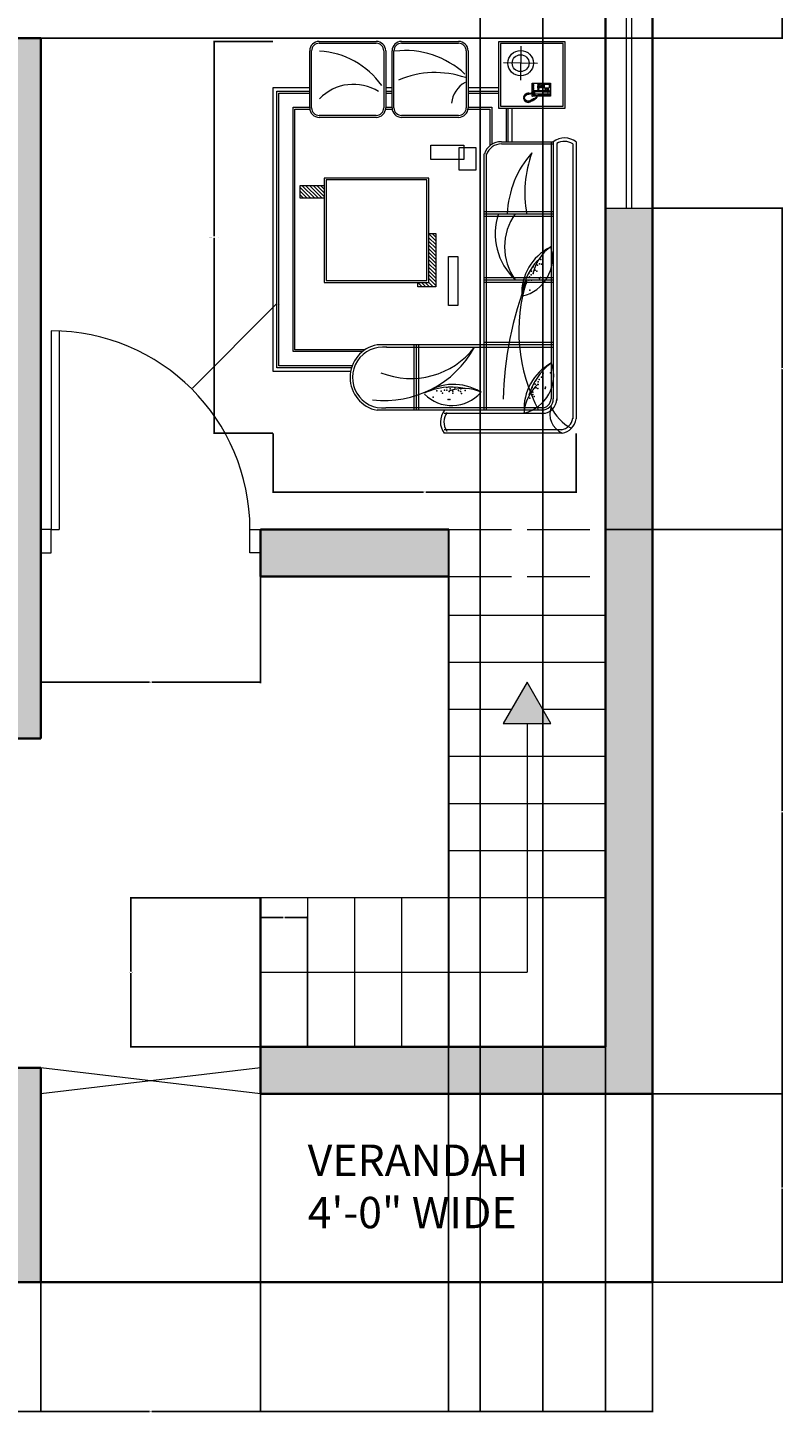
# Model space of a CAD drawing. Units: inches. Extents: x 126 to 477, y -70 to 465.
# Tile 2 of 5: x 332 to 477, y -70 to 195. Entities that reach past the tile are written whole.
import ezdxf

# ---------------------------------------------------------------- set-up
doc = ezdxf.new("R2010")
doc.units = ezdxf.units.IN
doc.linetypes.add('ACAD_ISO02W100', pattern=[15, 12, -3])
for name, color, linetype, lineweight in [('A-ANNO-DIMS', 2, 'Continuous', 18), ('A-ANNO-SYMB', 7, 'Continuous', 18), ('A-AREA-IDEN', 7, 'Continuous', 20), ('A-DOOR', 4, 'Continuous', 20), ('A-DOOR-GATE', 4, 'Continuous', 20), ('A-FLOR-STRS', 7, 'Continuous', 18), ('A-FLOR-STRS-OVHD', 7, 'ACAD_ISO02W100', 18), ('A-FURN', 8, 'Continuous', 18), ('A-GLAZ', 4, 'Continuous', 18), ('A-WALL', 7, 'Continuous', 35), ('A-WALL-PATT', 252, 'Continuous', 13)]:
    doc.layers.add(name, color=color, linetype=linetype, lineweight=lineweight)
doc.styles.get("Standard").update_dxf_attribs({"font": 'arial.ttf'})
doc.dimstyles.get("Standard").update_dxf_attribs({"dimtxt": 0.18, "dimasz": 0.18, "dimexe": 0.18, "dimexo": 0.0625, "dimgap": 0.09, "dimtad": 0, "dimtih": 1, "dimtoh": 1, "dimdec": 4, "dimzin": 0, "dimdsep": 46, "dimtxsty": 'Standard', "dimcen": 0.09, "dimadec": 0, "dimazin": 0, "dimtfac": 1, "dimtdec": 4, "dimtofl": 0, "dimtmove": 0, "dimatfit": 3, "dimfxl": 1, "dimtolj": 1, "dimtzin": 0, "dimarcsym": 0})

# ---------------------------------------------------------------- blocks, each defined once
blk = doc.blocks.new('A$C327A19D4')
for p, q in [((703, 3073), (3, 3073)), ((3, 3073), (3, 2373)), ((703, 2373), (703, 3073)), ((1059, 3191), (3976, 3191)), ((1078, 3155), (3976, 3155)), ((683, 3053), (23, 3053)), ((23, 3053), (23, 2393)), ((683, 2393), (683, 3053)), ((1056, 2949), (3763, 2949)), ((1056, 2403), (1056, 2949)), ((1056, 2925), (3763, 2925)), ((1076, 2985), (3780, 2985)), ((1080, 2403), (1080, 2949)), ((1791, 2223), (1791, 2949)), ((1815, 2465), (1815, 2949)), ((1839, 2223), (1839, 2949)), ((2487, 2223), (2487, 2949)), ((2511, 2223), (2511, 2949)), ((2535, 2223), (2535, 2949)), ((3169, 2223), (3169, 2949)), ((3193, 2465), (3193, 2949)), ((3221, 1195), (3221, 2949)), ((4090, 3043), (4090, 1800)), ((4126, 3043), (4126, 1800)), ((231, 2784), (227, 2425)), ((1815, 2223), (1815, 2872)), ((1815, 2223), (1815, 2872)), ((1815, 2465), (1815, 2872)), ((1815, 2465), (1815, 2872)), ((3193, 2223), (3193, 2872)), ((3193, 2223), (3193, 2872)), ((3193, 2465), (3193, 2872)), ((3193, 2465), (3193, 2872)), ((3860, 2828), (3860, 1185)), ((3884, 2828), (3884, 1095)), ((3920, 2867), (3920, 1802)), ((49, 2607), (409, 2603)), ((703, 2512), (1056, 2512)), ((3, 2373), (703, 2373)), ((23, 2393), (683, 2393)), ((484, 2052), (484, 2373)), ((524, 2052), (524, 2373)), ((544, 2052), (544, 2373)), ((703, 2472), (1056, 2472)), ((703, 2452), (1056, 2452)), ((694, 2052), (694, 2302)), ((694, 2302), (1084, 2302)), ((714, 2051), (714, 2282)), ((714, 2282), (1098, 2282)), ((3884, 2247), (1184, 2247)), ((3884, 2223), (1184, 2223)), ((3195, 2235), (3195, 1095)), ((1119, 2135), (1357, 2135)), ((1119, 1958), (1119, 2135)), ((1357, 2135), (1357, 1958)), ((1092, 2007), (1244, 2007)), ((1092, 1659), (1092, 2007)), ((1357, 1958), (1119, 1958)), ((1244, 2007), (1244, 1659)), ((2265, 1945), (2780, 1945)), ((2265, 1845), (2265, 1945)), ((2780, 1945), (2780, 1845)), ((2780, 1845), (2265, 1845)), ((1244, 1659), (1092, 1659)), ((2539, 1638), (1439, 1638)), ((1439, 1638), (1439, 538)), ((2519, 1618), (1459, 1618)), ((1459, 1618), (1459, 558)), ((2023, 1638), (2023, 1711)), ((2023, 1711), (2585, 1711)), ((2519, 558), (2519, 1618)), ((2539, 538), (2539, 1638)), ((2585, 1711), (2585, 1522)), ((2585, 1522), (2539, 1522)), ((3884, 1532), (3195, 1532)), ((3884, 1508), (3195, 1508)), ((3884, 1484), (3195, 1484)), ((484, 1185), (484, 1252)), ((524, 1185), (524, 1252)), ((544, 1185), (544, 1252)), ((694, 1185), (694, 1252)), ((714, 1184), (714, 1253)), ((3247, 967), (3247, 230)), ((3267, 940), (3267, 210)), ((3417, 832), (3417, 60)), ((3437, 825), (3437, 40)), ((3477, 816), (3477, 0)), ((1439, 538), (2539, 538)), ((1459, 558), (2519, 558)), ((1516, 538), (1651, 538)), ((1516, 285), (1516, 538)), ((1651, 538), (1651, 285)), ((484, 0), (484, 385)), ((524, 40), (524, 385)), ((544, 60), (544, 385)), ((694, 210), (694, 385)), ((714, 230), (714, 386)), ((3267, 210), (694, 210)), ((3247, 230), (714, 230)), ((1651, 285), (1516, 285)), ((3437, 40), (524, 40)), ((3417, 60), (544, 60)), ((3477, 0), (484, 0))]:
    blk.add_line(p, q)
at = {"linetype": 'ByBlock'}
for p, q in [((438, 2915), (440, 2918)), ((440, 2918), (576, 2919)), ((576, 2919), (578, 2916)), ((439, 2728), (438, 2915)), ((451, 2906), (490, 2906)), ((451, 2856), (451, 2906)), ((491, 2856), (451, 2856)), ((453, 2831), (453, 2839)), ((453, 2839), (461, 2839)), ((461, 2831), (453, 2831)), ((453, 2824), (461, 2825)), ((453, 2816), (453, 2824)), ((461, 2816), (453, 2816)), ((453, 2801), (453, 2810)), ((453, 2810), (461, 2810)), ((461, 2802), (453, 2801)), ((453, 2787), (453, 2795)), ((453, 2795), (461, 2795)), ((461, 2787), (453, 2787)), ((461, 2839), (461, 2831)), ((461, 2825), (461, 2816)), ((461, 2810), (461, 2802)), ((461, 2795), (461, 2787)), ((466, 2839), (475, 2840)), ((467, 2831), (466, 2839)), ((475, 2831), (467, 2831)), ((467, 2816), (467, 2825)), ((467, 2825), (475, 2825)), ((475, 2817), (467, 2816)), ((467, 2802), (467, 2810)), ((467, 2810), (475, 2810)), ((475, 2802), (467, 2802)), ((467, 2787), (467, 2795)), ((467, 2795), (475, 2795)), ((475, 2787), (467, 2787)), ((475, 2840), (475, 2831)), ((475, 2825), (475, 2817)), ((475, 2810), (475, 2802)), ((475, 2795), (475, 2787)), ((480, 2840), (488, 2840)), ((480, 2831), (480, 2840)), ((488, 2832), (480, 2831)), ((480, 2817), (480, 2825)), ((480, 2825), (488, 2825)), ((488, 2817), (480, 2817)), ((480, 2810), (488, 2810)), ((480, 2802), (480, 2810)), ((488, 2802), (480, 2802)), ((480, 2787), (480, 2795)), ((480, 2795), (488, 2795)), ((488, 2787), (480, 2787)), ((488, 2840), (488, 2832)), ((488, 2825), (488, 2817)), ((488, 2810), (488, 2802)), ((488, 2795), (488, 2787)), ((490, 2906), (491, 2856)), ((505, 2903), (494, 2903)), ((494, 2903), (494, 2899)), ((494, 2899), (505, 2899)), ((495, 2895), (495, 2891)), ((505, 2895), (495, 2895)), ((495, 2891), (505, 2891)), ((495, 2887), (495, 2883)), ((505, 2887), (495, 2887)), ((495, 2883), (505, 2883)), ((495, 2879), (495, 2875)), ((505, 2879), (495, 2879)), ((495, 2875), (505, 2875)), ((495, 2871), (495, 2867)), ((506, 2871), (495, 2871)), ((495, 2867), (506, 2867)), ((495, 2863), (495, 2859)), ((506, 2863), (495, 2863)), ((495, 2859), (506, 2859)), ((497, 2795), (507, 2795)), ((497, 2787), (497, 2795)), ((507, 2787), (497, 2787)), ((505, 2899), (505, 2903)), ((505, 2891), (505, 2895)), ((505, 2883), (505, 2887)), ((505, 2875), (505, 2879)), ((506, 2867), (506, 2871)), ((506, 2859), (506, 2863)), ((507, 2795), (507, 2787)), ((515, 2908), (520, 2914)), ((516, 2744), (515, 2908)), ((520, 2910), (519, 2905)), ((519, 2905), (531, 2893)), ((519, 2905), (519, 2868)), ((519, 2868), (522, 2862)), ((520, 2914), (561, 2915)), ((526, 2913), (520, 2910)), ((520, 2783), (522, 2790)), ((520, 2746), (520, 2783)), ((522, 2862), (526, 2855)), ((522, 2790), (526, 2797)), ((532, 2895), (526, 2913)), ((526, 2913), (558, 2913)), ((526, 2855), (527, 2845)), ((526, 2797), (528, 2806)), ((527, 2845), (527, 2832)), ((528, 2806), (527, 2832)), ((531, 2893), (532, 2895)), ((532, 2832), (531, 2893)), ((551, 2896), (532, 2895)), ((532, 2832), (532, 2759)), ((551, 2896), (558, 2913)), ((553, 2893), (551, 2896)), ((565, 2905), (553, 2893)), ((553, 2832), (553, 2893)), ((553, 2832), (554, 2759)), ((558, 2855), (557, 2846)), ((557, 2846), (557, 2832)), ((557, 2806), (557, 2832)), ((559, 2797), (557, 2806)), ((558, 2913), (563, 2911)), ((562, 2862), (558, 2855)), ((563, 2790), (559, 2797)), ((561, 2915), (568, 2908)), ((565, 2869), (562, 2862)), ((563, 2911), (565, 2905)), ((566, 2783), (563, 2790)), ((565, 2905), (565, 2869)), ((566, 2747), (566, 2783)), ((568, 2908), (569, 2745)), ((578, 2916), (580, 2729)), ((587, 2779), (579, 2779)), ((579, 2775), (584, 2774)), ((584, 2774), (587, 2772)), ((590, 2777), (587, 2779)), ((587, 2772), (591, 2770)), ((594, 2771), (590, 2777)), ((599, 2771), (594, 2771)), ((602, 2770), (599, 2771)), ((442, 2726), (439, 2728)), ((543, 2726), (442, 2726)), ((468, 2743), (455, 2743)), ((455, 2743), (455, 2735)), ((455, 2735), (469, 2735)), ((469, 2735), (468, 2743)), ((487, 2743), (474, 2743)), ((474, 2743), (474, 2735)), ((474, 2735), (487, 2735)), ((487, 2735), (487, 2743)), ((493, 2744), (493, 2735)), ((506, 2744), (493, 2744)), ((493, 2735), (506, 2735)), ((506, 2735), (506, 2744)), ((523, 2737), (516, 2744)), ((520, 2746), (532, 2759)), ((521, 2741), (520, 2746)), ((527, 2738), (521, 2741)), ((542, 2737), (523, 2737)), ((533, 2756), (527, 2738)), ((527, 2738), (542, 2738)), ((532, 2759), (533, 2756)), ((552, 2756), (533, 2756)), ((546, 2743), (542, 2743)), ((542, 2743), (542, 2731)), ((542, 2731), (545, 2717)), ((545, 2717), (549, 2704)), ((547, 2732), (546, 2743)), ((546, 2738), (559, 2739)), ((562, 2737), (546, 2737)), ((549, 2696), (546, 2692)), ((546, 2692), (546, 2686)), ((546, 2686), (554, 2685)), ((554, 2685), (546, 2680)), ((546, 2680), (547, 2672)), ((548, 2723), (547, 2732)), ((547, 2672), (555, 2672)), ((577, 2726), (548, 2726)), ((552, 2710), (548, 2723)), ((549, 2704), (548, 2697)), ((548, 2697), (549, 2696)), ((555, 2672), (548, 2666)), ((548, 2666), (551, 2659)), ((551, 2659), (560, 2661)), ((554, 2759), (552, 2756)), ((552, 2756), (559, 2739)), ((553, 2703), (552, 2710)), ((552, 2696), (553, 2703)), ((557, 2693), (552, 2696)), ((566, 2747), (554, 2759)), ((556, 2687), (557, 2693)), ((558, 2669), (556, 2687)), ((560, 2661), (556, 2653)), ((556, 2653), (560, 2648)), ((568, 2656), (558, 2669)), ((559, 2739), (565, 2741)), ((560, 2648), (566, 2653)), ((569, 2745), (562, 2737)), ((565, 2741), (566, 2747)), ((566, 2653), (565, 2646)), ((565, 2646), (570, 2642)), ((583, 2649), (568, 2656)), ((570, 2642), (577, 2648)), ((577, 2648), (576, 2639)), ((576, 2639), (582, 2637)), ((580, 2729), (577, 2726)), ((582, 2637), (585, 2645)), ((599, 2647), (583, 2649)), ((585, 2645), (589, 2637)), ((589, 2637), (593, 2637)), ((591, 2770), (593, 2768)), ((595, 2768), (592, 2765)), ((592, 2765), (597, 2757)), ((593, 2768), (595, 2768)), ((593, 2637), (595, 2645)), ((595, 2645), (598, 2636)), ((597, 2757), (606, 2742)), ((598, 2636), (604, 2637)), ((599, 2760), (603, 2767)), ((606, 2763), (599, 2760)), ((615, 2654), (599, 2647)), ((603, 2767), (602, 2770)), ((604, 2750), (608, 2758)), ((612, 2753), (604, 2750)), ((604, 2645), (610, 2639)), ((604, 2637), (604, 2645)), ((608, 2758), (606, 2763)), ((606, 2742), (612, 2731)), ((608, 2742), (614, 2749)), ((615, 2746), (608, 2742)), ((610, 2639), (615, 2642)), ((614, 2749), (612, 2753)), ((612, 2731), (614, 2730)), ((613, 2733), (618, 2740)), ((621, 2736), (613, 2733)), ((614, 2730), (613, 2728)), ((613, 2728), (622, 2712)), ((614, 2650), (619, 2643)), ((615, 2642), (614, 2650)), ((618, 2740), (615, 2746)), ((627, 2666), (615, 2654)), ((619, 2643), (624, 2647)), ((620, 2723), (624, 2730)), ((627, 2725), (620, 2723)), ((620, 2654), (628, 2651)), ((624, 2647), (620, 2654)), ((624, 2730), (621, 2736)), ((622, 2712), (631, 2687)), ((626, 2712), (630, 2720)), ((634, 2713), (626, 2712)), ((630, 2720), (627, 2725)), ((631, 2687), (627, 2666)), ((628, 2702), (636, 2705)), ((637, 2702), (628, 2702)), ((628, 2661), (636, 2659)), ((632, 2654), (628, 2661)), ((628, 2651), (632, 2654)), ((631, 2672), (640, 2672)), ((638, 2665), (631, 2672)), ((633, 2691), (639, 2696)), ((641, 2691), (633, 2691)), ((636, 2705), (634, 2713)), ((634, 2681), (642, 2684)), ((641, 2677), (634, 2681)), ((636, 2659), (638, 2665)), ((639, 2696), (637, 2702)), ((640, 2672), (641, 2677)), ((642, 2684), (641, 2691))]:
    blk.add_line(p, q, dxfattribs=at)
at = {"ltscale": 5}
for p, q in [((100, 2052), (700, 2052)), ((0, 1352), (0, 1952)), ((20, 1352), (20, 1952)), ((100, 2032), (700, 2032)), ((780, 1952), (780, 1352)), ((800, 1952), (800, 1352)), ((2023, 1673), (2061, 1711)), ((2027, 1638), (2100, 1711)), ((2067, 1638), (2139, 1711)), ((2106, 1638), (2179, 1711)), ((2145, 1638), (2218, 1711)), ((2184, 1638), (2257, 1711)), ((2224, 1638), (2296, 1711)), ((2263, 1638), (2336, 1711)), ((2302, 1638), (2375, 1711)), ((2341, 1638), (2414, 1711)), ((2381, 1638), (2453, 1711)), ((2420, 1638), (2493, 1711)), ((2459, 1638), (2532, 1711)), ((2498, 1638), (2571, 1711)), ((2538, 1638), (2585, 1685)), ((2539, 1601), (2585, 1646)), ((2539, 1561), (2585, 1607)), ((2539, 1522), (2585, 1568)), ((2578, 1522), (2585, 1528)), ((700, 1272), (100, 1272)), ((700, 1252), (100, 1252)), ((100, 1185), (700, 1185)), ((0, 485), (0, 1085)), ((20, 485), (20, 1085)), ((100, 1165), (700, 1165)), ((780, 1085), (780, 485)), ((800, 1085), (800, 485)), ((1516, 499), (1555, 538)), ((1516, 460), (1594, 538)), ((1516, 421), (1634, 538)), ((1516, 382), (1651, 516)), ((1516, 342), (1651, 477)), ((1516, 303), (1651, 438)), ((700, 405), (100, 405)), ((700, 385), (100, 385)), ((1537, 285), (1651, 398)), ((1576, 285), (1651, 359)), ((1616, 285), (1651, 320))]:
    blk.add_line(p, q, dxfattribs=at)
for radius in [134, 88.7]:
    blk.add_circle((229, 2605), radius)
for centre, radius, start, end in [((1218, 3068), 201, 142.4201, 216.3682), ((1218, 3068), 165, 148.4003, 210.2229), ((3657, 3353), 468, 293.6733, 332.9672), ((3943, 3007), 150, 10.9855, 79.893), ((3943, 3007), 187, 10.9855, 79.893), ((2545, 3192), 468, 214.7097, 257.8799), ((2283, 2531), 409, 13.4523, 105.9639), ((3869, 3188), 547, 208.8478, 273.48), ((3911, 3323), 657, 217.6007, 253.5739), ((3517, 2544), 409, 14.6876, 107.1992), ((3763, 2828), 157, 0, 90), ((3763, 2828), 121, 0, 90), ((3763, 2828), 96.8, 0, 90), ((3921, 3138), 226, 250.4844, 335.1673), ((2657, 3163), 547, 207.1715, 271.8037), ((2752, 3267), 657, 227.0776, 263.0508), ((3052, 4350), 1764, 252.1519, 298.1592), ((3951, 3106), 468, 222.7716, 265.9418), ((1594, 3859), 1211, 249.7283, 280.5443), ((1853, 3485), 1021, 228.2765, 267.8541), ((3865, 6197), 3777, 248.9971, 268.5461), ((2024, 3008), 670, 251.8392, 316.629), ((2163, 3036), 599, 234.5154, 305.4846), ((1243, 2401), 187, 179.2584, 251.6848), ((1243, 2401), 163, 179.2584, 251.6848), ((4124, 2008), 468, 156.691, 199.8613), ((4159, 1898), 547, 149.1529, 213.7851), ((3425, 1881), 409, 315.4337, 47.9453), ((4298, 1873), 657, 169.059, 205.0321), ((4007, 1962), 201, 232.4201, 306.3682), ((4007, 1962), 165, 232.4201, 306.3682)]:
    blk.add_arc(centre, radius, start, end)
for centre, radius, start, end in [((100, 1952), 100, 90, 180), ((700, 1952), 100, 0, 90), ((100, 1952), 80, 90, 180), ((1024, 1388), 928, 137.1341, 186.5635), ((1307, 1706), 979, 160.9364, 203.1944), ((676, 2156), 279, 209.1633, 264.4137), ((700, 1952), 80, 0, 90), ((100, 1352), 100, 180, 270), ((100, 1352), 80, 180, 270), ((700, 1352), 80, 270, 0), ((700, 1352), 100, 270, 0), ((100, 1085), 100, 90, 180), ((700, 1085), 100, 0, 90), ((100, 1085), 80, 90, 180), ((968, 436), 868, 125.4807, 176.5616), ((949, 846), 497, 147.8484, 226.1244), ((700, 1085), 80, 0, 90), ((100, 485), 100, 180, 270), ((100, 485), 80, 180, 270), ((700, 485), 100, 270, 0), ((700, 485), 80, 270, 0)]:
    blk.add_arc(centre, radius, start, end, dxfattribs=at)
at = {"ltscale": 20}
for centre, radius, start, end in [((2701, 1449), 849, 338.2682, 52.2695), ((2703, 1175), 1078, 353.1988, 61.2564), ((3540, 1156), 321, 172.9078, 5.2194), ((3540, 1161), 351, 190.8398, 349.1602)]:
    blk.add_arc(centre, radius, start, end, dxfattribs=at)
for p in [(3492, 2920), (2298, 2818), (2329, 2780), (2344, 2802), (2345, 2825), (2356, 2781), (2421, 2774), (2485, 2814), (2498, 2803), (3495, 2842), (3535, 2825), (3560, 2838), (3561, 2800), (3585, 2789), (3612, 2788), (3641, 2868), (3655, 2787), (3657, 2862), (2375, 2736), (2410, 2757), (2421, 2720), (2444, 2738), (2445, 2691), (2459, 2715), (2481, 2700), (2514, 2718), (2515, 2690), (2551, 2664), (2620, 2701), (3571, 2765), (3609, 2758), (3646, 2728), (3647, 2768), (3694, 2735), (3707, 2710), (3719, 2734), (3738, 2747), (3756, 2703), (3648, 1911), (3660, 1974), (3676, 1951), (3677, 2020), (3687, 1973), (3707, 1984), (3646, 1828), (3658, 1864), (3673, 1803), (3674, 1829), (3683, 1768), (3684, 1893), (3686, 1853), (3705, 1892), (3706, 1784), (3770, 1842), (3772, 1859), (3680, 1724), (3748, 1685)]:
    blk.add_point(p)
blk = doc.blocks.new('WIN-72IN')
for p, q in [((0, 0), (0, 9)), ((72, 0), (72, 9)), ((72, 5), (0, 5)), ((72, 4), (0, 4))]:
    blk.add_line(p, q)
blk = doc.blocks.new('*D25')
at = {"layer": 'A-ANNO-DIMS', "color": 0, "lineweight": -2, "transparency": 16777216}
for p, q in [((378.9, 192.26), (367.54, 192.26)), ((367.72, 192.08), (367.72, 154.96)), ((367.72, 117.47), (367.72, 154.59)), ((378.9, 117.29), (367.54, 117.29))]:
    blk.add_line(p, q, dxfattribs=at)
at = {"layer": 'A-ANNO-DIMS', "color": 0, "transparency": 16777216}
for points in [[(367.69, 192.08), (367.75, 192.08), (367.72, 192.26)], [(367.69, 117.47), (367.75, 117.47), (367.72, 117.29)]]:
    blk.add_solid(points, dxfattribs=at)
at = {"layer": 'Defpoints', "color": 0, "transparency": 16777216}
for p in [(378.96, 192.26), (367.72, 117.29), (378.96, 117.29)]:
    blk.add_point(p, dxfattribs=at)
at = {"layer": 'A-ANNO-DIMS', "color": 0, "transparency": 16777216, "insert": (367.72, 154.77), "char_height": 0.18, "attachment_point": 5}
blk.add_mtext('\\A1;LOUNGE SET 75', dxfattribs=at)
blk = doc.blocks.new('*D26')
at = {"layer": 'A-ANNO-DIMS', "color": 0, "lineweight": -2, "transparency": 16777216}
for p, q in [((378.96, 117.23), (378.96, 105.86)), ((436.94, 117.23), (436.94, 105.86)), ((379.14, 106.04), (407.73, 106.04)), ((436.76, 106.04), (408.17, 106.04))]:
    blk.add_line(p, q, dxfattribs=at)
at = {"layer": 'A-ANNO-DIMS', "color": 0, "transparency": 16777216}
for points in [[(379.14, 106.07), (379.14, 106.01), (378.96, 106.04)], [(436.76, 106.07), (436.76, 106.01), (436.94, 106.04)]]:
    blk.add_solid(points, dxfattribs=at)
at = {"layer": 'Defpoints', "color": 0, "transparency": 16777216}
for p in [(378.96, 117.29), (436.94, 117.29), (436.94, 106.04)]:
    blk.add_point(p, dxfattribs=at)
at = {"layer": 'A-ANNO-DIMS', "color": 0, "transparency": 16777216, "insert": (407.95, 106.04), "char_height": 0.18, "attachment_point": 5}
blk.add_mtext('\\A1;58', dxfattribs=at)
blk = doc.blocks.new('*D32')
at = {"layer": 'A-ANNO-DIMS', "color": 0, "lineweight": -2, "transparency": 16777216}
for p, q in [((430.53, 430.82), (430.53, -70.05)), ((442.53, 430.82), (442.53, -70.05)), ((430.71, -69.87), (436.32, -69.87)), ((442.35, -69.87), (436.74, -69.87))]:
    blk.add_line(p, q, dxfattribs=at)
at = {"layer": 'A-ANNO-DIMS', "color": 0, "transparency": 16777216}
for points in [[(430.71, -69.84), (430.71, -69.9), (430.53, -69.87)], [(442.35, -69.84), (442.35, -69.9), (442.53, -69.87)]]:
    blk.add_solid(points, dxfattribs=at)
at = {"layer": 'Defpoints', "color": 0, "transparency": 16777216}
for p in [(430.53, 430.88), (442.53, 430.88), (442.53, -69.87)]:
    blk.add_point(p, dxfattribs=at)
at = {"layer": 'A-ANNO-DIMS', "color": 0, "transparency": 16777216, "insert": (436.53, -69.87), "char_height": 0.18, "attachment_point": 5}
blk.add_mtext('\\A1;12', dxfattribs=at)
blk = doc.blocks.new('*D34')
at = {"layer": 'A-ANNO-DIMS', "color": 0, "lineweight": -2, "transparency": 16777216}
for p, q in [((451.6, -9.12), (476.46, -9.12)), ((476.28, -9.3), (476.28, -26.94)), ((476.28, -44.94), (476.28, -27.3)), ((451.6, -45.12), (476.46, -45.12))]:
    blk.add_line(p, q, dxfattribs=at)
at = {"layer": 'A-ANNO-DIMS', "color": 0, "transparency": 16777216}
for points in [[(476.25, -9.3), (476.31, -9.3), (476.28, -9.12)], [(476.25, -44.94), (476.31, -44.94), (476.28, -45.12)]]:
    blk.add_solid(points, dxfattribs=at)
at = {"layer": 'Defpoints', "color": 0, "transparency": 16777216}
for p in [(451.53, -9.12), (476.28, -9.12), (451.53, -45.12)]:
    blk.add_point(p, dxfattribs=at)
at = {"layer": 'A-ANNO-DIMS', "color": 0, "transparency": 16777216, "insert": (476.28, -27.12), "char_height": 0.18, "attachment_point": 5}
blk.add_mtext('\\A1;36', dxfattribs=at)
blk = doc.blocks.new('*D35')
at = {"layer": 'A-ANNO-DIMS', "color": 0, "lineweight": -2, "transparency": 16777216}
for p, q in [((442.6, 98.88), (476.46, 98.88)), ((476.28, 98.7), (476.28, 45.06)), ((476.28, -8.94), (476.28, 44.7)), ((451.6, -9.12), (476.46, -9.12))]:
    blk.add_line(p, q, dxfattribs=at)
at = {"layer": 'A-ANNO-DIMS', "color": 0, "transparency": 16777216}
for points in [[(476.25, 98.7), (476.31, 98.7), (476.28, 98.88)], [(476.25, -8.94), (476.31, -8.94), (476.28, -9.12)]]:
    blk.add_solid(points, dxfattribs=at)
at = {"layer": 'Defpoints', "color": 0, "transparency": 16777216}
for p in [(442.53, 98.88), (476.28, 98.88), (451.53, -9.12)]:
    blk.add_point(p, dxfattribs=at)
at = {"layer": 'A-ANNO-DIMS', "color": 0, "transparency": 16777216, "insert": (476.28, 44.88), "char_height": 0.18, "attachment_point": 5}
blk.add_mtext('\\A1;108', dxfattribs=at)
blk = doc.blocks.new('*D36')
at = {"layer": 'A-ANNO-DIMS', "color": 0, "lineweight": -2, "transparency": 16777216}
for p, q in [((451.6, 160.38), (476.46, 160.38)), ((476.28, 160.2), (476.28, 129.81)), ((476.28, 99.06), (476.28, 129.45)), ((442.6, 98.88), (476.46, 98.88))]:
    blk.add_line(p, q, dxfattribs=at)
at = {"layer": 'A-ANNO-DIMS', "color": 0, "transparency": 16777216}
for points in [[(476.25, 160.2), (476.31, 160.2), (476.28, 160.38)], [(476.25, 99.06), (476.31, 99.06), (476.28, 98.88)]]:
    blk.add_solid(points, dxfattribs=at)
at = {"layer": 'Defpoints', "color": 0, "transparency": 16777216}
for p in [(451.53, 160.38), (476.28, 160.38), (442.53, 98.88)]:
    blk.add_point(p, dxfattribs=at)
at = {"layer": 'A-ANNO-DIMS', "color": 0, "transparency": 16777216, "insert": (476.28, 129.63), "char_height": 0.18, "attachment_point": 5}
blk.add_mtext('\\A1;61.5', dxfattribs=at)
blk = doc.blocks.new('*D40')
at = {"layer": 'A-ANNO-DIMS', "color": 0, "lineweight": -2, "transparency": 16777216}
for p, q in [((317.53, -45.18), (317.53, -70.05)), ((334.53, -45.18), (334.53, -70.05)), ((317.71, -69.87), (325.82, -69.87)), ((334.35, -69.87), (326.24, -69.87))]:
    blk.add_line(p, q, dxfattribs=at)
at = {"layer": 'A-ANNO-DIMS', "color": 0, "transparency": 16777216}
for points in [[(317.71, -69.84), (317.71, -69.9), (317.53, -69.87)], [(334.35, -69.84), (334.35, -69.9), (334.53, -69.87)]]:
    blk.add_solid(points, dxfattribs=at)
at = {"layer": 'Defpoints', "color": 0, "transparency": 16777216}
for p in [(317.53, -45.12), (334.53, -45.12), (334.53, -69.87)]:
    blk.add_point(p, dxfattribs=at)
at = {"layer": 'A-ANNO-DIMS', "color": 0, "transparency": 16777216, "insert": (326.03, -69.87), "char_height": 0.18, "attachment_point": 5}
blk.add_mtext('\\A1;17', dxfattribs=at)
blk = doc.blocks.new('*D41')
at = {"layer": 'A-ANNO-DIMS', "color": 0, "lineweight": -2, "transparency": 16777216}
for p, q in [((334.53, -4.18), (334.53, -70.05)), ((376.53, -9.18), (376.53, -70.05)), ((334.71, -69.87), (355.31, -69.87)), ((376.35, -69.87), (355.75, -69.87))]:
    blk.add_line(p, q, dxfattribs=at)
at = {"layer": 'A-ANNO-DIMS', "color": 0, "transparency": 16777216}
for points in [[(334.71, -69.84), (334.71, -69.9), (334.53, -69.87)], [(376.35, -69.84), (376.35, -69.9), (376.53, -69.87)]]:
    blk.add_solid(points, dxfattribs=at)
at = {"layer": 'Defpoints', "color": 0, "transparency": 16777216}
for p in [(334.53, -4.12), (376.53, -9.12), (376.53, -69.87)]:
    blk.add_point(p, dxfattribs=at)
at = {"layer": 'A-ANNO-DIMS', "color": 0, "transparency": 16777216, "insert": (355.53, -69.87), "char_height": 0.18, "attachment_point": 5}
blk.add_mtext('\\A1;42', dxfattribs=at)
blk = doc.blocks.new('*D42')
at = {"layer": 'A-ANNO-DIMS', "color": 0, "lineweight": -2, "transparency": 16777216}
for p, q in [((376.53, -9.18), (376.53, -70.05)), ((451.53, -9.18), (451.53, -70.05)), ((376.71, -69.87), (413.81, -69.87)), ((451.35, -69.87), (414.25, -69.87))]:
    blk.add_line(p, q, dxfattribs=at)
at = {"layer": 'A-ANNO-DIMS', "color": 0, "transparency": 16777216}
for points in [[(376.71, -69.84), (376.71, -69.9), (376.53, -69.87)], [(451.35, -69.84), (451.35, -69.9), (451.53, -69.87)]]:
    blk.add_solid(points, dxfattribs=at)
at = {"layer": 'Defpoints', "color": 0, "transparency": 16777216}
for p in [(376.53, -9.12), (451.53, -9.12), (451.53, -69.87)]:
    blk.add_point(p, dxfattribs=at)
at = {"layer": 'A-ANNO-DIMS', "color": 0, "transparency": 16777216, "insert": (414.03, -69.87), "char_height": 0.18, "attachment_point": 5}
blk.add_mtext('\\A1;75', dxfattribs=at)
blk = doc.blocks.new('*D43')
at = {"layer": 'A-ANNO-DIMS', "color": 0, "lineweight": -2, "transparency": 16777216}
for p, q in [((412.53, 98.82), (412.53, -70.05)), ((442.53, 98.82), (442.53, -70.05)), ((412.71, -69.87), (427.31, -69.87)), ((442.35, -69.87), (427.75, -69.87))]:
    blk.add_line(p, q, dxfattribs=at)
at = {"layer": 'A-ANNO-DIMS', "color": 0, "transparency": 16777216}
for points in [[(412.71, -69.84), (412.71, -69.9), (412.53, -69.87)], [(442.35, -69.84), (442.35, -69.9), (442.53, -69.87)]]:
    blk.add_solid(points, dxfattribs=at)
at = {"layer": 'Defpoints', "color": 0, "transparency": 16777216}
for p in [(412.53, 98.88), (442.53, 98.88), (442.53, -69.87)]:
    blk.add_point(p, dxfattribs=at)
at = {"layer": 'A-ANNO-DIMS', "color": 0, "transparency": 16777216, "insert": (427.53, -69.87), "char_height": 0.18, "attachment_point": 5}
blk.add_mtext('\\A1;30', dxfattribs=at)
blk = doc.blocks.new('*D44')
at = {"layer": 'A-ANNO-DIMS', "color": 0, "lineweight": -2, "transparency": 16777216}
for p, q in [((376.47, 28.4), (351.6, 28.4)), ((351.78, 28.22), (351.78, 14.32)), ((351.78, 0.06), (351.78, 13.96)), ((376.47, -0.12), (351.6, -0.12))]:
    blk.add_line(p, q, dxfattribs=at)
at = {"layer": 'A-ANNO-DIMS', "color": 0, "transparency": 16777216}
for points in [[(351.75, 28.22), (351.81, 28.22), (351.78, 28.4)], [(351.75, 0.06), (351.81, 0.06), (351.78, -0.12)]]:
    blk.add_solid(points, dxfattribs=at)
at = {"layer": 'Defpoints', "color": 0, "transparency": 16777216}
for p in [(351.78, 28.4), (376.53, 28.4), (376.53, -0.12)]:
    blk.add_point(p, dxfattribs=at)
at = {"layer": 'A-ANNO-DIMS', "color": 0, "transparency": 16777216, "insert": (351.78, 14.14), "char_height": 0.18, "attachment_point": 5}
blk.add_mtext('\\A1;28.524', dxfattribs=at)
blk = doc.blocks.new('*D45')
at = {"layer": 'A-ANNO-DIMS', "color": 0, "lineweight": -2, "transparency": 16777216}
for p, q in [((376.53, -0.06), (376.53, 24.81)), ((376.71, 24.63), (380.88, 24.63)), ((385.35, 24.63), (381.18, 24.63)), ((385.53, -0.06), (385.53, 24.81))]:
    blk.add_line(p, q, dxfattribs=at)
at = {"layer": 'A-ANNO-DIMS', "color": 0, "transparency": 16777216}
for points in [[(376.71, 24.66), (376.71, 24.6), (376.53, 24.63)], [(385.35, 24.66), (385.35, 24.6), (385.53, 24.63)]]:
    blk.add_solid(points, dxfattribs=at)
at = {"layer": 'Defpoints', "color": 0, "transparency": 16777216}
for p in [(385.53, 24.63), (376.53, -0.12), (385.53, -0.12)]:
    blk.add_point(p, dxfattribs=at)
at = {"layer": 'A-ANNO-DIMS', "color": 0, "transparency": 16777216, "insert": (381.03, 24.63), "char_height": 0.18, "attachment_point": 5}
blk.add_mtext('\\A1;9', dxfattribs=at)
blk = doc.blocks.new('*D47')
at = {"layer": 'A-ANNO-DIMS', "color": 0, "lineweight": -2, "transparency": 16777216}
for p, q in [((334.53, 94.32), (334.53, 69.45)), ((376.53, 94.32), (376.53, 69.45)), ((334.71, 69.63), (355.31, 69.63)), ((376.35, 69.63), (355.75, 69.63))]:
    blk.add_line(p, q, dxfattribs=at)
at = {"layer": 'A-ANNO-DIMS', "color": 0, "transparency": 16777216}
for points in [[(334.71, 69.66), (334.71, 69.6), (334.53, 69.63)], [(376.35, 69.66), (376.35, 69.6), (376.53, 69.63)]]:
    blk.add_solid(points, dxfattribs=at)
at = {"layer": 'Defpoints', "color": 0, "transparency": 16777216}
for p in [(334.53, 94.38), (376.53, 94.38), (334.53, 69.63)]:
    blk.add_point(p, dxfattribs=at)
at = {"layer": 'A-ANNO-DIMS', "color": 0, "transparency": 16777216, "insert": (355.53, 69.63), "char_height": 0.18, "attachment_point": 5}
blk.add_mtext('\\A1;42', dxfattribs=at)
blk = doc.blocks.new('*D48')
at = {"layer": 'A-ANNO-DIMS', "color": 0, "lineweight": -2, "transparency": 16777216}
for p, q in [((418.53, 298.82), (418.53, -70.05)), ((442.53, 298.82), (442.53, -70.05)), ((418.71, -69.87), (430.31, -69.87)), ((442.35, -69.87), (430.75, -69.87))]:
    blk.add_line(p, q, dxfattribs=at)
at = {"layer": 'A-ANNO-DIMS', "color": 0, "transparency": 16777216}
for points in [[(418.71, -69.84), (418.71, -69.9), (418.53, -69.87)], [(442.35, -69.84), (442.35, -69.9), (442.53, -69.87)]]:
    blk.add_solid(points, dxfattribs=at)
at = {"layer": 'Defpoints', "color": 0, "transparency": 16777216}
for p in [(418.53, 298.88), (442.53, 298.88), (442.53, -69.87)]:
    blk.add_point(p, dxfattribs=at)
at = {"layer": 'A-ANNO-DIMS', "color": 0, "transparency": 16777216, "insert": (430.53, -69.87), "char_height": 0.18, "attachment_point": 5}
blk.add_mtext('\\A1;24', dxfattribs=at)
blk = doc.blocks.new('*D51')
at = {"layer": 'A-ANNO-DIMS', "color": 0, "lineweight": -2, "transparency": 16777216}
for p, q in [((293.6, 222.88), (476.46, 222.88)), ((476.28, 222.7), (476.28, 208.06)), ((476.28, 193.06), (476.28, 207.7)), ((293.6, 192.88), (476.46, 192.88))]:
    blk.add_line(p, q, dxfattribs=at)
at = {"layer": 'A-ANNO-DIMS', "color": 0, "transparency": 16777216}
for points in [[(476.25, 222.7), (476.31, 222.7), (476.28, 222.88)], [(476.25, 193.06), (476.31, 193.06), (476.28, 192.88)]]:
    blk.add_solid(points, dxfattribs=at)
at = {"layer": 'Defpoints', "color": 0, "transparency": 16777216}
for p in [(293.53, 222.88), (476.28, 222.88), (293.53, 192.88)]:
    blk.add_point(p, dxfattribs=at)
at = {"layer": 'A-ANNO-DIMS', "color": 0, "transparency": 16777216, "insert": (476.28, 207.88), "char_height": 0.18, "attachment_point": 5}
blk.add_mtext('\\A1;30', dxfattribs=at)
blk = doc.blocks.new('*D58')
at = {"layer": 'A-ANNO-DIMS', "color": 0, "lineweight": -2, "transparency": 16777216}
for p, q in [((379.5, 141.9), (363.52, 125.89)), ((379.68, 141.9), (379.5, 141.9)), ((336.44, 98.88), (336.62, 98.88)), ((336.53, 98.79), (336.53, 98.97))]:
    blk.add_line(p, q, dxfattribs=at)
at = {"layer": 'A-ANNO-DIMS', "color": 0, "transparency": 16777216}
blk.add_solid([(363.5, 125.91), (363.54, 125.87), (363.39, 125.77)], dxfattribs=at)
at = {"layer": 'Defpoints', "color": 0, "transparency": 16777216}
for p in [(363.39, 125.77), (336.53, 98.88)]:
    blk.add_point(p, dxfattribs=at)
at = {"layer": 'A-ANNO-DIMS', "color": 0, "transparency": 16777216, "insert": (379.99, 141.9), "char_height": 0.18, "attachment_point": 5}
blk.add_mtext('\\A1;R38', dxfattribs=at)

msp = doc.modelspace()

# ---------------------------------------------------------------- hatches: boundary and pattern name
at = {"layer": 'A-ANNO-SYMB'}
h = msp.add_hatch(color=256, dxfattribs=at)
h.dxf.hatch_style = 1
h.paths.add_polyline_path([(427.5333, 69.6737), (422.9704, 61.7705), (432.0962, 61.7705)])
at = {"layer": 'A-WALL-PATT'}
h = msp.add_hatch(color=256, dxfattribs=at)
h.dxf.hatch_style = 1
h.paths.add_polyline_path([(334.5333, -4.1194), (329.5333, -4.1194), (329.5333, -40.1194), (317.5333, -40.1194), (317.5333, -45.1194), (334.5333, -45.1194)])
h.paths.add_polyline_path([(205.5333, 58.8806), (233.5333, 58.8806), (233.5333, 67.8806), (209.5333, 67.8806), (209.5333, 187.8806), (293.5333, 187.8806), (293.5333, 192.8806), (209.5333, 192.8806), (209.5333, 204.8806), (200.5333, 204.8806), (200.5333, -45.1194), (209.5333, -45.1194), (209.5333, -40.1194), (205.5333, -40.1194)])
h = msp.add_hatch(color=256, dxfattribs=at)
h.dxf.hatch_style = 1
h.paths.add_polyline_path([(334.5333, 192.8806), (329.5333, 192.8806), (329.5333, 67.8806), (305.5333, 67.8806), (305.5333, 58.8806), (334.5333, 58.8806)])
h = msp.add_hatch(color=256, dxfattribs=at)
h.dxf.hatch_style = 1
h.paths.add_polyline_path([(451.5333, 160.3806), (442.5333, 160.3806), (442.5333, 98.8806), (442.5333, -0.1194), (376.5333, -0.1194), (376.5333, -1.5951), (376.5333, -9.1194), (451.5333, -9.1194)])
h = msp.add_hatch(color=256, dxfattribs=at)
h.dxf.hatch_style = 1
h.paths.add_polyline_path([(412.5333, 98.8806), (376.5333, 98.8806), (376.5333, 89.8806), (412.5333, 89.8806)])

# ---------------------------------------------------------------- linework, layer by layer
at = {"layer": 'A-ANNO-SYMB'}
for p in [(427.5333, 61.7705), (376.5333, 14.1428)]:
    msp.add_line(p, (427.5333, 14.1428), dxfattribs=at)
msp.add_lwpolyline([(427.5333, 69.6737), (422.9704, 61.7705), (432.0962, 61.7705)], close=True, dxfattribs=at)
at = {"layer": 'A-DOOR'}
for p, q in [((336.5333, 136.8806), (336.5333, 98.8806)), ((338.0333, 136.851), (338.0333, 98.8806)), ((336.5333, 98.8806), (334.5333, 98.8806)), ((336.5333, 94.3806), (336.5333, 98.8806)), ((336.5333, 98.8806), (338.0333, 98.8806)), ((374.5333, 94.3806), (374.5333, 98.8806)), ((374.5333, 98.8806), (376.5333, 98.8806)), ((334.5333, 94.3806), (336.5333, 94.3806)), ((376.5333, 94.3806), (374.5333, 94.3806))]:
    msp.add_line(p, q, dxfattribs=at)
msp.add_arc((336.5333, 98.8806), 38, 0.059331, 90, dxfattribs=at)
at = {"layer": 'A-DOOR-GATE'}
for p, q in [((376.5333, -4.1194), (334.5333, -9.1194)), ((376.5333, -9.1194), (334.5333, -4.1194))]:
    msp.add_line(p, q, dxfattribs=at)
at = {"layer": 'A-FLOR-STRS'}
for p, q in [((412.5333, 98.8806), (412.5333, -0.1194)), ((442.5333, 82.4049), (412.5333, 82.4049)), ((442.5333, 73.4049), (412.5333, 73.4049)), ((424.4914, 64.4049), (412.5333, 64.4049)), ((442.5333, 64.4049), (430.5752, 64.4049)), ((442.5333, 55.4049), (412.5333, 55.4049)), ((442.5333, 46.4049), (412.5333, 46.4049)), ((442.5333, 37.4049), (412.5333, 37.4049)), ((442.5333, 28.4049), (376.5333, 28.4049)), ((385.5333, 28.4049), (385.5333, -0.1194)), ((394.5333, 28.4049), (394.5333, -0.1194)), ((403.5333, 28.4049), (403.5333, -0.1194))]:
    msp.add_line(p, q, dxfattribs=at)
at = {"layer": 'A-FLOR-STRS-OVHD'}
for p, q in [((412.5333, 98.8806), (442.5333, 98.8806)), ((412.5333, 89.8806), (442.5333, 89.8806))]:
    msp.add_line(p, q, dxfattribs=at)
at = {"layer": 'A-WALL'}
for p, q in [((451.5333, 439.8806), (451.5333, -45.1194)), ((442.5333, 293.8806), (442.5333, 98.8806)), ((329.5333, 192.8806), (334.5333, 192.8806)), ((334.5333, 58.8806), (334.5333, 192.8806)), ((376.5333, 98.8806), (412.5333, 98.8806)), ((376.5333, 98.8806), (376.5333, 89.8806)), ((442.5333, 98.8806), (442.5333, -0.1194)), ((376.5333, 89.8806), (412.5333, 89.8806)), ((205.5333, 58.8806), (334.5333, 58.8806)), ((376.5333, 28.4049), (376.5333, -1.5951)), ((376.5333, 28.4049), (376.5333, -9.1194)), ((376.5333, -0.1194), (442.5333, -0.1194)), ((334.5333, -4.1194), (329.5333, -4.1194)), ((334.5333, -4.1194), (334.5333, -45.1194)), ((376.5333, -9.1194), (451.5333, -9.1194)), ((317.5333, -45.1194), (451.5333, -45.1194))]:
    msp.add_line(p, q, dxfattribs=at)

# ---------------------------------------------------------------- block references
at = {"layer": 'A-FURN', "xscale": 0.0181684437462713, "yscale": 0.0181684437462713, "zscale": 0.0181684437462713, "rotation": 270}
msp.add_blockref('A$C327A19D4', (378.9637, 192.2559), dxfattribs=at)
at = {"layer": 'A-GLAZ', "rotation": 269.9999999999998}
msp.add_blockref('WIN-72IN', (442.5333, 232.3806), dxfattribs=at)

# ---------------------------------------------------------------- texts
at = {"layer": 'A-AREA-IDEN', "insert": (385.5762, -18.8273), "char_height": 6, "attachment_point": 1}
msp.add_mtext_dynamic_manual_height_columns('VERANDAH\\P4\'-0" WIDE', width=64.633583, gutter_width=12.5, heights=[0], dxfattribs=at)

# ---------------------------------------------------------------- dimensions: what is measured, and where the dimension line sits
at = {"layer": 'A-ANNO-DIMS'}
for base, p1, p2, picture, middle in [((442.5333, -69.8694), (430.5333, 430.8806), (442.5333, 430.8806), '*D32', (436.5333, -69.8694)), ((442.5333, -69.8694), (418.5333, 298.8806), (442.5333, 298.8806), '*D48', (430.5333, -69.8694)), ((436.9395, 106.0445), (378.9637, 117.2894), (436.9395, 117.2894), '*D26', (407.9516, 106.0445)), ((442.5333, -69.8694), (412.5333, 98.8806), (442.5333, 98.8806), '*D43', (427.5333, -69.8694)), ((385.5333, 24.6306), (376.5333, -0.1194), (385.5333, -0.1194), '*D45', (381.0333, 24.6306)), ((376.5333, -69.8694), (334.5333, -4.1194), (376.5333, -9.1194), '*D41', (355.5333, -69.8694)), ((451.5333, -69.8694), (376.5333, -9.1194), (451.5333, -9.1194), '*D42', (414.0333, -69.8694)), ((334.5333, -69.8694), (317.5333, -45.1194), (334.5333, -45.1194), '*D40', (326.0333, -69.8694))]:
    dim = msp.add_linear_dim(base=base, p1=p1, p2=p2, dimstyle='Standard', override={"dimdec": 0, "dimlfac": 1, "dimrnd": 0, "dimzin": 0, "dimdsep": 46, "dimlunit": 2}, dxfattribs=at)
    dim.commit()
    dim.dimension.update_dxf_attribs({"geometry": picture, "text_midpoint": middle})
for base, p1, p2, angle, override, picture, middle in [((476.2833, 222.8806), (293.5333, 192.8806), (293.5333, 222.8806), 90, {"dimdec": 0, "dimlfac": 1, "dimrnd": 0, "dimzin": 0, "dimdsep": 46, "dimlunit": 2}, '*D51', (476.2833, 207.8806)), ((476.2833, 160.3806), (442.5333, 98.8806), (451.5333, 160.3806), 90, {"dimdec": 1, "dimlfac": 1, "dimrnd": 0, "dimzin": 0, "dimdsep": 46, "dimlunit": 2}, '*D36', (476.2833, 129.6306)), ((476.2833, 98.8806), (451.5333, -9.1194), (442.5333, 98.8806), 90, {"dimdec": 0, "dimlfac": 1, "dimrnd": 0, "dimzin": 0, "dimdsep": 46, "dimlunit": 2}, '*D35', (476.2833, 44.8806)), ((334.5333, 69.6306), (376.5333, 94.3806), (334.5333, 94.3806), 180, {"dimdec": 0, "dimlfac": 1, "dimrnd": 0, "dimzin": 0, "dimdsep": 46, "dimlunit": 2}, '*D47', (355.5333, 69.6306)), ((351.7833, 28.4049), (376.5333, -0.1194), (376.5333, 28.4049), 90, {"dimdec": 3, "dimlfac": 1, "dimrnd": 0, "dimzin": 0, "dimdsep": 46, "dimlunit": 2}, '*D44', (351.7833, 14.1428)), ((476.2833, -9.1194), (451.5333, -45.1194), (451.5333, -9.1194), 90, {"dimdec": 0, "dimlfac": 1, "dimrnd": 0, "dimzin": 0, "dimdsep": 46, "dimlunit": 2}, '*D34', (476.2833, -27.1194))]:
    dim = msp.add_linear_dim(base=base, p1=p1, p2=p2, angle=angle, dimstyle='Standard', override=override, dxfattribs=at)
    dim.commit()
    dim.dimension.update_dxf_attribs({"geometry": picture, "text_midpoint": middle})
dim = msp.add_linear_dim(base=(367.7188, 117.2894), p1=(378.9637, 192.2559), p2=(378.9637, 117.2894), angle=270, text='LOUNGE SET <>', dimstyle='Standard', override={"dimdec": 0, "dimlfac": 1, "dimrnd": 0, "dimzin": 0, "dimdsep": 46, "dimlunit": 2}, dxfattribs=at)
dim.commit()
dim.dimension.update_dxf_attribs({"geometry": '*D25', "text_midpoint": (367.7188, 154.7727)})
dim = msp.add_radius_dim(center=(336.5333, 98.8806), mpoint=(363.389, 125.765), dimstyle='Standard', override={"dimdec": 0, "dimlfac": 1, "dimrnd": 0, "dimzin": 0, "dimdsep": 46, "dimlunit": 2}, dxfattribs=at)
dim.commit()
dim.dimension.update_dxf_attribs({"geometry": '*D58', "text_midpoint": (379.9877, 141.8957), "dimtype": 164})

doc.saveas('drawing.dxf')
